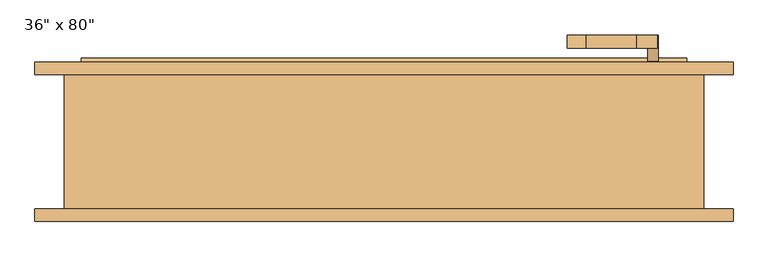
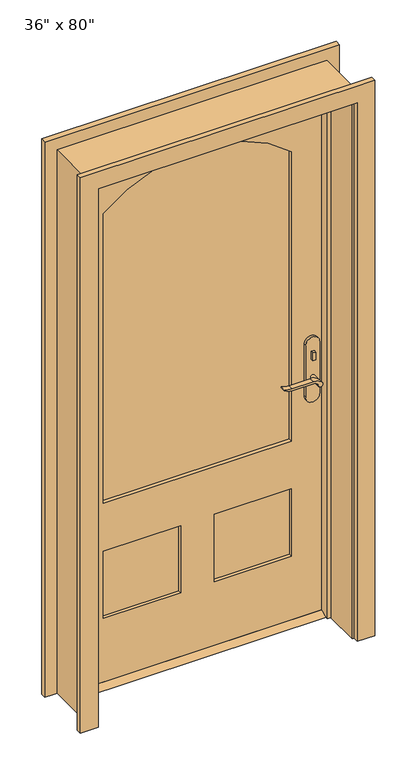
"""IFC4 building model written with IfcOpenShell, lengths in millimetres: door geometry."""

from ifc_helpers import new_model, si_unit, point, frame, frame_2d, origin, place, context, project, spatial, polyline, circle_curve, trimmed, segment, composite_curve, outline, extrude, faceted_brep, source, transform, mapped, element, save


def door_1768e003(model_context):
    return source(origin(), model_context, "Body", "SolidModel", [
        extrude(outline(polyline([(63.5, 12.7), (98.425, 12.7), (123.825, 0.0), (38.1, 0.0), (63.5, 12.7)])), frame((-457.2, 0.0, 0.0), z_axis=(1.0, 0.0, 0.0), x_axis=(0.0, 1.0, 0.0)), (0.0, 0.0, 1.0), 914.4),
        extrude(outline(polyline([(411.4, 43.5), (401.4, 43.5), (401.4, 53.5), (411.4, 53.5), (411.4, 43.5)])), frame((0.0, 0.0, 981.9), z_axis=(0.0, 0.0, 1.0), x_axis=(1.0, 0.0, 0.0)), (0.0, 0.0, 1.0), 30.0),
        extrude(outline(composite_curve([segment(trimmed(circle_curve(frame_2d((996.9, 406.4)), 8.0), [point((996.9, 398.4))], [point((996.9, 414.4))], False, "CARTESIAN"), True, "CONTINUOUS"), segment(trimmed(circle_curve(frame_2d((996.9, 406.4)), 8.0), [point((996.9, 414.4))], [point((996.9, 398.4))], False, "CARTESIAN"), True, "CONTINUOUS")], self_intersect=False)), frame((0.0, 108.425, 0.0), z_axis=(0.0, 1.0, 0.0), x_axis=(0.0, 0.0, 1.0)), (0.0, 0.0, 1.0), 10.0),
        extrude(outline(composite_curve([segment(trimmed(circle_curve(frame_2d((897.1555521, 382.7324871)), 37.2832219), [point((919.0523287, 412.9081363))], [point((934.4, 381.0325667))], False, "CARTESIAN"), True, "CONTINUOUS"), segment(polyline([(934.4, 381.0325667), (934.4, 304.7564091)]), True, "CONTINUOUS"), segment(trimmed(circle_curve(frame_2d((1017.6850638, 304.8227909)), 83.2850902), [point((934.4, 304.7564091))], [point((939.4, 276.4))], True, "CARTESIAN"), True, "CONTINUOUS"), segment(polyline([(939.4, 276.4), (936.6135558, 276.4)]), True, "CONTINUOUS"), segment(trimmed(circle_curve(frame_2d((986.6709207, 308.3396612)), 59.3791355), [point((936.6135558, 276.4))], [point((927.4, 304.7564091))], False, "CARTESIAN"), True, "CONTINUOUS"), segment(polyline([(927.4, 304.7564091), (927.4, 381.0138099)]), True, "CONTINUOUS"), segment(trimmed(circle_curve(frame_2d((909.2738613, 381.0138099)), 18.1261387), [point((927.4, 381.0138099))], [point((914.4, 398.4))], True, "CARTESIAN"), True, "CONTINUOUS"), segment(trimmed(circle_curve(frame_2d((914.4, 406.4)), 8.0), [point((914.4, 398.4))], [point((919.0523287, 412.9081363))], False, "CARTESIAN"), True, "CONTINUOUS")], self_intersect=False)), frame((0.0, 3.5, 0.0), z_axis=(0.0, 1.0, 0.0), x_axis=(0.0, 0.0, 1.0)), (0.0, 0.0, 1.0), 20.0),
        extrude(outline(composite_curve([segment(trimmed(circle_curve(frame_2d((914.4, 406.4)), 8.0), [point((914.3999903, 398.4))], [point((919.0523287, 412.9081363))], False, "CARTESIAN"), True, "CONTINUOUS"), segment(trimmed(circle_curve(frame_2d((897.1555521, 382.7324871)), 37.2832219), [point((919.0523287, 412.9081363))], [point((934.4, 381.0325667))], False, "CARTESIAN"), True, "CONTINUOUS"), segment(polyline([(934.4, 381.0325667), (934.4, 304.7564091)]), True, "CONTINUOUS"), segment(trimmed(circle_curve(frame_2d((1017.6850638, 304.8227909)), 83.2850902), [point((934.4, 304.7564091))], [point((939.4, 276.4))], True, "CARTESIAN"), True, "CONTINUOUS"), segment(polyline([(939.4, 276.4), (936.6135558, 276.4)]), True, "CONTINUOUS"), segment(trimmed(circle_curve(frame_2d((986.6709207, 308.3396612)), 59.3791355), [point((936.6135558, 276.4))], [point((927.4, 304.7564091))], False, "CARTESIAN"), True, "CONTINUOUS"), segment(polyline([(927.4, 304.7564091), (927.4, 381.0138122)]), True, "CONTINUOUS"), segment(trimmed(circle_curve(frame_2d((909.2738682, 381.0138122)), 18.1261318), [point((927.4, 381.0138122))], [point((914.3999903, 398.4))], True, "CARTESIAN"), True, "CONTINUOUS")], self_intersect=False)), frame((0.0, 138.425, 0.0), z_axis=(0.0, 1.0, 0.0), x_axis=(0.0, 0.0, 1.0)), (0.0, 0.0, 1.0), 20.0),
        extrude(outline(composite_curve([segment(trimmed(circle_curve(frame_2d((914.4, 406.4)), 8.0), [point((914.4, 398.4))], [point((914.4, 414.4))], False, "CARTESIAN"), True, "CONTINUOUS"), segment(trimmed(circle_curve(frame_2d((914.4, 406.4)), 8.0), [point((914.4, 414.4))], [point((914.4, 398.4))], False, "CARTESIAN"), True, "CONTINUOUS")], self_intersect=False)), frame((0.0, 23.5, 0.0), z_axis=(0.0, 1.0, 0.0), x_axis=(0.0, 0.0, 1.0)), (0.0, 0.0, 1.0), 30.0),
        extrude(outline(composite_curve([segment(trimmed(circle_curve(frame_2d((914.4, 406.4)), 8.0), [point((914.4, 398.4))], [point((914.4, 414.4))], False, "CARTESIAN"), True, "CONTINUOUS"), segment(trimmed(circle_curve(frame_2d((914.4, 406.4)), 8.0), [point((914.4, 414.4))], [point((914.4, 398.4))], False, "CARTESIAN"), True, "CONTINUOUS")], self_intersect=False)), frame((0.0, 108.425, 0.0), z_axis=(0.0, 1.0, 0.0), x_axis=(0.0, 0.0, 1.0)), (0.0, 0.0, 1.0), 30.0),
        extrude(outline(composite_curve([segment(polyline([(844.4, 431.4), (1039.4, 431.4)]), True, "CONTINUOUS"), segment(trimmed(circle_curve(frame_2d((1039.4, 406.4)), 25.0), [point((1039.4, 431.4))], [point((1039.4, 381.4))], False, "CARTESIAN"), True, "CONTINUOUS"), segment(polyline([(1039.4, 381.4), (844.4, 381.4)]), True, "CONTINUOUS"), segment(trimmed(circle_curve(frame_2d((844.4, 406.4)), 25.0), [point((844.4, 381.4))], [point((844.4, 431.4))], False, "CARTESIAN"), True, "CONTINUOUS")], self_intersect=False)), frame((0.0, 53.5, 0.0), z_axis=(0.0, 1.0, 0.0), x_axis=(0.0, 0.0, 1.0)), (0.0, 0.0, 1.0), 10.0),
        extrude(outline(composite_curve([segment(polyline([(844.4, 431.4), (1039.4, 431.4)]), True, "CONTINUOUS"), segment(trimmed(circle_curve(frame_2d((1039.4, 406.4)), 25.0), [point((1039.4, 431.4))], [point((1039.4, 381.4))], False, "CARTESIAN"), True, "CONTINUOUS"), segment(polyline([(1039.4, 381.4), (844.4, 381.4)]), True, "CONTINUOUS"), segment(trimmed(circle_curve(frame_2d((844.4, 406.4)), 25.0), [point((844.4, 381.4))], [point((844.4, 431.4))], False, "CARTESIAN"), True, "CONTINUOUS")], self_intersect=False)), frame((0.0, 98.425, 0.0), z_axis=(0.0, 1.0, 0.0), x_axis=(0.0, 0.0, 1.0)), (0.0, 0.0, 1.0), 10.0),
        extrude(outline(polyline([(2032.0, -457.2), (12.7, -457.2), (12.7, 457.2), (2032.0, 457.2), (2032.0, -457.2)]), holes=[composite_curve([segment(polyline([(688.975, -336.55), (1784.35, -336.55)]), True, "CONTINUOUS"), segment(trimmed(circle_curve(frame_2d((1401.92125, 0.0)), 509.42875), [point((1784.35, -336.55))], [point((1784.35, 336.55))], True, "CARTESIAN"), True, "CONTINUOUS"), segment(polyline([(1784.35, 336.55), (688.975, 336.55), (688.975, -336.55)]), True, "CONTINUOUS")], self_intersect=False), polyline([(508.0, -60.325), (254.0, -60.325), (254.0, -336.55), (508.0, -336.55), (508.0, -60.325)]), polyline([(508.0, 336.55), (254.0, 336.55), (254.0, 60.325), (508.0, 60.325), (508.0, 336.55)])]), frame((0.0, 63.5, 0.0), z_axis=(0.0, 1.0, 0.0), x_axis=(0.0, 0.0, 1.0)), (0.0, 0.0, 1.0), 34.925),
        faceted_brep([(482.6, 98.425, 0.0), (482.6, -104.775, 0.0), (457.2, -104.775, 0.0), (457.2, 28.575, 0.0), (444.5, 28.575, 0.0), (444.5, 63.5, 0.0), (457.2, 63.5, 0.0), (457.2, 98.425, 0.0), (482.6, 98.425, 2057.4), (482.6, -104.775, 2057.4), (-482.6, -104.775, 2057.4), (-482.6, -104.775, 0.0), (-457.2, -104.775, 0.0), (-457.2, -104.775, 2032.0), (457.2, -104.775, 2032.0), (457.2, 28.575, 2032.0), (-457.2, 28.575, 2032.0), (-457.2, 28.575, 0.0), (-444.5, 28.575, 0.0), (-444.5, 28.575, 2019.3), (444.5, 28.575, 2019.3), (444.5, 63.5, 2019.3), (-444.5, 63.5, 2019.3), (-444.5, 63.5, 0.0), (-457.2, 63.5, 0.0), (-457.2, 63.5, 2032.0), (457.2, 63.5, 2032.0), (457.2, 98.425, 2032.0), (-457.2, 98.425, 2032.0), (-457.2, 98.425, 0.0), (-482.6, 98.425, 0.0), (-482.6, 98.425, 2057.4)], [[[0, 1, 2, 3, 4, 5, 6, 7]], [[1, 0, 8, 9]], [[2, 1, 9, 10, 11, 12, 13, 14]], [[3, 2, 14, 15]], [[4, 3, 15, 16, 17, 18, 19, 20]], [[5, 4, 20, 21]], [[6, 5, 21, 22, 23, 24, 25, 26]], [[7, 6, 26, 27]], [[0, 7, 27, 28, 29, 30, 31, 8]], [[9, 8, 31, 10]], [[15, 14, 13, 16]], [[21, 20, 19, 22]], [[27, 26, 25, 28]], [[30, 29, 24, 23, 18, 17, 12, 11]], [[10, 31, 30, 11]], [[16, 13, 12, 17]], [[22, 19, 18, 23]], [[28, 25, 24, 29]]]),
        extrude(outline(polyline([(-60.325, 75.1416667), (-336.55, 75.1416667), (-336.55, 86.7833333), (-60.325, 86.7833333), (-60.325, 75.1416667)])), frame((0.0, 0.0, 254.0), z_axis=(0.0, 0.0, 1.0), x_axis=(1.0, 0.0, 0.0)), (0.0, 0.0, 1.0), 254.0),
        extrude(outline(polyline([(336.55, 75.1416667), (60.325, 75.1416667), (60.325, 86.7833333), (336.55, 86.7833333), (336.55, 75.1416667)])), frame((0.0, 0.0, 254.0), z_axis=(0.0, 0.0, 1.0), x_axis=(1.0, 0.0, 0.0)), (0.0, 0.0, 1.0), 254.0),
        extrude(outline(composite_curve([segment(polyline([(688.975, -336.55), (688.975, 336.55), (1784.35, 336.55)]), True, "CONTINUOUS"), segment(trimmed(circle_curve(frame_2d((1401.92125, 0.0)), 509.42875), [point((1784.35, 336.55))], [point((1784.35, -336.55))], False, "CARTESIAN"), True, "CONTINUOUS"), segment(polyline([(1784.35, -336.55), (688.975, -336.55)]), True, "CONTINUOUS")], self_intersect=False)), frame((0.0, 77.47, 0.0), z_axis=(0.0, 1.0, 0.0), x_axis=(0.0, 0.0, 1.0)), (0.0, 0.0, 1.0), 6.985),
        extrude(outline(polyline([(0.0, -527.05), (0.0, -463.55), (2038.35, -463.55), (2038.35, 463.55), (0.0, 463.55), (0.0, 527.05), (2101.85, 527.05), (2101.85, -527.05), (0.0, -527.05)])), frame((0.0, -123.825, 0.0), z_axis=(0.0, 1.0, 0.0), x_axis=(0.0, 0.0, 1.0)), (0.0, 0.0, 1.0), 19.05),
        extrude(outline(polyline([(0.0, -527.05), (0.0, -463.55), (2038.35, -463.55), (2038.35, 463.55), (0.0, 463.55), (0.0, 527.05), (2101.85, 527.05), (2101.85, -527.05), (0.0, -527.05)])), frame((0.0, 98.425, 0.0), z_axis=(0.0, 1.0, 0.0), x_axis=(0.0, 0.0, 1.0)), (0.0, 0.0, 1.0), 19.05),
    ])


if __name__ == "__main__":
    model = new_model("IFC4")
    model_context = context("Model", 3, world=origin())
    ifc_project = project(units=[si_unit("LENGTHUNIT", "METRE", prefix="MILLI")], contexts=[model_context])
    site = spatial("IfcSite", under=ifc_project)
    building = spatial("IfcBuilding", under=site)
    placement = place(None, origin())
    door_shape = door_1768e003(model_context)
    element("IfcDoor", 1, ObjectType="36\" x 80\"", at=placement, inside=building, context=model_context, shape_type="MappedRepresentation", body=[
        mapped(door_shape, transform((0.0, 0.0, 0.0), x_axis=(1.0, 0.0, 0.0), y_axis=(0.0, 1.0, 0.0), z_axis=(0.0, 0.0, 1.0))),
    ])
    save(model, "model.ifc")

# Revit data of these elements
# Type "36\" x 80\""
#   Type Mark = "8"
#   Assembly Code = "B2030100"
#   Analytic Construction = "French door, wood frame with single glass"
#   Threshold Offset [instance default] = 0' - 0 1/2"
#   Thickness = 0' - 1 3/8"
#   Thermal Resistance (R) = 1.0696 (h·ft²·°F)/BTU
#   Swing Angle [instance default] = 90.00°
#   Stiles = 0' - 4 3/4"
#   Rough Width = 3' - 2"
#   Rough Height = 6' - 9"
#   Radius = 1' - 8.05625"
#   Lock Rail = 0' - 7 1/8"
#   Height = 6' - 8"
#   Width = 3' - 0"
#   Heat Transfer Coefficient (U) = 0.9350 BTU/(h·ft²·°F)
#   Door Offset [instance default] = 0' - 0"
#   Bottom Rail = 0' - 9 1/2"
#   Threshold [instance default] = yes
#   Function = 1
#   Exterior Trim [instance default] = yes
#   Trim Material = Cherry
#   Threshold Material = Cherry
#   Panel Material = Cherry
#   Glazing = Glass
#   Frame Material = Cherry
#   Door Handle Material = Aluminum
#   Visual Light Transmittance = 0
#   Solar Heat Gain Coefficient = 0
#   Wall Closure = (empty or 0)
#   Construction Type = (empty or 0)
# Element 1 (IfcDoor, "36\" x 80\"")
#   Materials on its faces: "Cherry", "Aluminum", "Glass"
# Materials
#   "Cherry": class "Wood", colour RGB 226 177 128, transparency 0, Description = "Prunus Serotina", Cost = 0
#   "Glass": class "Glass", colour RGB 0 128 192, transparency 0.75, Description = "Soda Lime Glass", Cost = 0
#   "Aluminum": class "Metal", colour RGB 247 247 247, transparency 0, Description = "Aluminum 6061", Cost = 0
